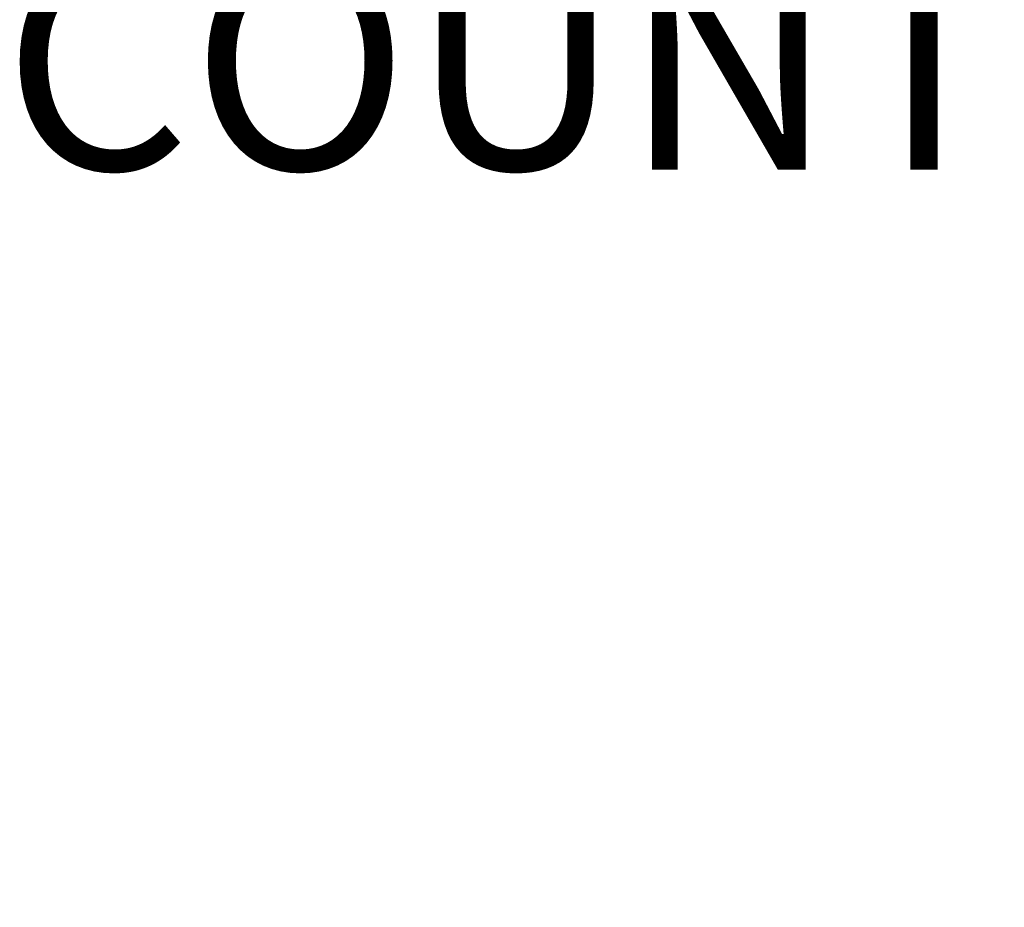
# Model space of a CAD drawing. Units: inches. Extents: x -1198 to -69, y -512 to 437.
# Tile 39 of 50: x -637 to -610, y 186 to 210. Entities that reach past the tile are written whole.
import ezdxf

# ---------------------------------------------------------------- set-up
doc = ezdxf.new("R2010")
doc.units = ezdxf.units.IN
doc.header["$MEASUREMENT"] = 0
doc.layers.add('A-ANNO-DIMS', color=2, linetype='Continuous', lineweight=18)
doc.styles.get("Standard").update_dxf_attribs({"font": 'arial.ttf'})
doc.dimstyles.get("Standard").update_dxf_attribs({"dimtxt": 6, "dimasz": 6, "dimexe": 0.18, "dimexo": 0.0625, "dimgap": 0.09, "dimtad": 0, "dimtih": 1, "dimtoh": 1, "dimdec": 0, "dimzin": 0, "dimdsep": 46, "dimlunit": 4, "dimtxsty": 'Standard', "dimblk": 'OBLIQUE', "dimcen": 0.09, "dimadec": 0, "dimazin": 0, "dimtfac": 1, "dimtdec": 0, "dimtofl": 0, "dimtmove": 0, "dimatfit": 3, "dimfxl": 1, "dimtolj": 1, "dimtzin": 0, "dimarcsym": 0})

# ---------------------------------------------------------------- blocks, each defined once
blk = doc.blocks.new('_Oblique')
at = {"color": 0, "linetype": 'ByBlock', "lineweight": -2}
blk.add_line((-0.5, -0.5), (0.5, 0.5), dxfattribs=at)
blk = doc.blocks.new('*D56')
at = {"layer": 'A-ANNO-DIMS', "color": 0, "lineweight": -2, "ltscale": 10, "transparency": 16777216}
for p, q in [((-618.339, 257.228), (-603.822, 257.228)), ((-604.002, 257.228), (-604.002, 212.422)), ((-604.002, 161.228), (-604.002, 206.033)), ((-618.339, 161.228), (-603.822, 161.228))]:
    blk.add_line(p, q, dxfattribs=at)
at = {"layer": 'DEFPOINTS', "color": 0, "ltscale": 10, "transparency": 16777216}
for p in [(-618.402, 257.228), (-604.002, 257.228), (-618.402, 161.228)]:
    blk.add_point(p, dxfattribs=at)
at = {"layer": 'A-ANNO-DIMS', "color": 0, "lineweight": -2, "ltscale": 10, "transparency": 16777216, "xscale": 6, "yscale": 6, "zscale": 6}
for p, rotation in [((-604.002, 257.228), 90), ((-604.002, 161.228), 270)]:
    blk.add_blockref('_Oblique', p, dxfattribs=dict(at, rotation=rotation))
at = {"layer": 'A-ANNO-DIMS', "color": 0, "ltscale": 10, "transparency": 16777216, "insert": (-604.002, 209.228), "char_height": 6, "attachment_point": 5}
blk.add_mtext('\\A1;COUNTER 96 TYP.', dxfattribs=at)

msp = doc.modelspace()

# ---------------------------------------------------------------- dimensions: what is measured, and where the dimension line sits
at = {"layer": 'A-ANNO-DIMS', "ltscale": 10}
dim = msp.add_linear_dim(base=(-604.0019, 257.2277), p1=(-618.4019, 161.2277), p2=(-618.4019, 257.2277), angle=90, text='COUNTER <> TYP.', dimstyle='Standard', override={"dimdec": 0, "dimlfac": 1, "dimrnd": 0, "dimzin": 0, "dimdsep": 46, "dimlunit": 2}, dxfattribs=at)
dim.commit()
dim.dimension.update_dxf_attribs({"geometry": '*D56', "text_midpoint": (-604.0019, 209.2277)})

doc.saveas('drawing.dxf')
